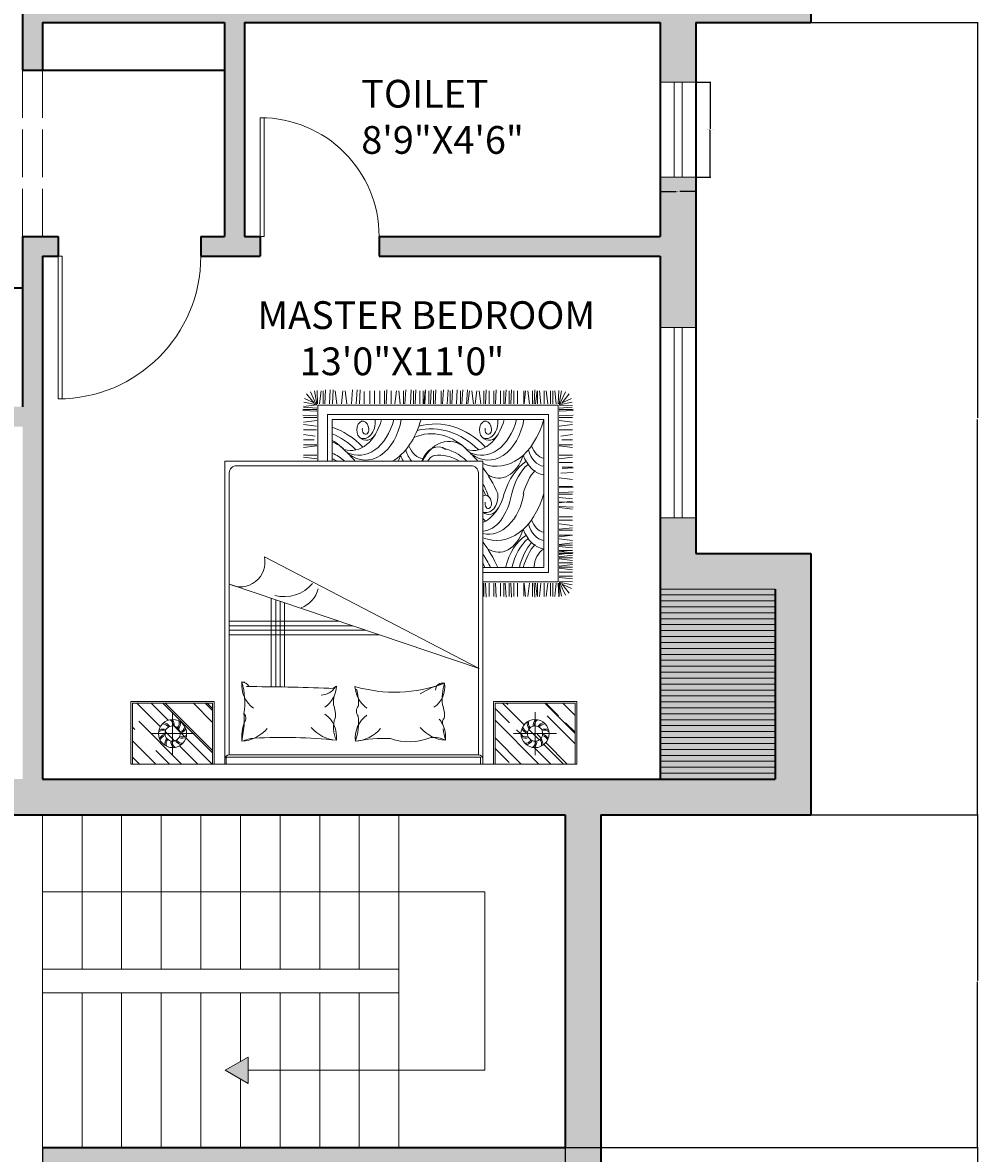
# Model space of a CAD drawing. Units: inches. Extents: x 2540 to 3167, y 3083 to 4007.
# Tile 14 of 15: x 2926 to 3167, y 3542 to 3828. Entities that reach past the tile are written whole.
import ezdxf

# ---------------------------------------------------------------- set-up
doc = ezdxf.new("R2010")
doc.units = ezdxf.units.IN
doc.linetypes.add('ACAD_ISO02W100', pattern=[15, 12, -3])
for name, color, linetype, lineweight in [('A-ANNO-DIMS', 2, 'Continuous', 18), ('A-ANNO-SYMB', 7, 'Continuous', 18), ('A-AREA-IDEN', 7, 'Continuous', 18), ('A-DOOR', 4, 'Continuous', 18), ('A-FLOR-PATT', 8, 'Continuous', 13), ('A-FLOR-STRS', 7, 'Continuous', 18), ('A-FURN', 8, 'Continuous', 13), ('A-GLAZ', 4, 'Continuous', 18)]:
    doc.layers.add(name, color=color, linetype=linetype, lineweight=lineweight)
for name, color, linetype, lineweight, true_color in [('A-WALL', 143, 'Continuous', 35, 0x7aafdf), ('A-WALL-OVHD', 143, 'ACAD_ISO02W100', 18, 0x7aafdf), ('A-WALL-PATT', 143, 'Continuous', 13, 0x7aafdf)]:
    doc.layers.add(name, color=color, linetype=linetype, lineweight=lineweight, true_color=true_color)
doc.styles.get("Standard").update_dxf_attribs({"font": 'arial.ttf'})
doc.dimstyles.get("Standard").update_dxf_attribs({"dimtxt": 0.18, "dimasz": 0.18, "dimexe": 0.18, "dimexo": 0.0625, "dimgap": 0.09, "dimtad": 0, "dimtih": 1, "dimtoh": 1, "dimdec": 4, "dimzin": 0, "dimdsep": 46, "dimtxsty": 'Standard', "dimcen": 0.09, "dimadec": 0, "dimazin": 0, "dimtfac": 1, "dimtdec": 4, "dimtofl": 0, "dimtmove": 0, "dimatfit": 3, "dimfxl": 1, "dimtolj": 1, "dimtzin": 0, "dimarcsym": 0})

# ---------------------------------------------------------------- blocks, each defined once
blk = doc.blocks.new('*U3')
blk.add_line((0, 0), (0, 29))
blk = doc.blocks.new('*U4')
at = {"layer": 'A-FLOR-PATT', "color": 0, "linetype": 'ByBlock', "lineweight": -2, "transparency": 16777216, "rotation": 270}
for p in [(3086.51, 3684.71), (3086.51, 3683.21), (3086.51, 3681.71), (3086.51, 3680.21), (3086.51, 3678.71), (3086.51, 3677.21), (3086.51, 3675.71), (3086.51, 3674.21), (3086.51, 3672.71), (3086.51, 3671.21), (3086.51, 3669.71), (3086.51, 3668.21), (3086.51, 3666.71), (3086.51, 3665.21), (3086.51, 3663.71), (3086.51, 3662.21), (3086.51, 3660.71), (3086.51, 3659.21), (3086.51, 3657.71), (3086.51, 3656.21), (3086.51, 3654.71), (3086.51, 3653.21), (3086.51, 3651.71), (3086.51, 3650.21), (3086.51, 3648.71), (3086.51, 3647.21), (3086.51, 3645.71), (3086.51, 3644.21), (3086.51, 3642.71), (3086.51, 3641.21), (3086.51, 3639.71), (3086.51, 3638.21), (3086.51, 3636.71)]:
    blk.add_blockref('*U3', p, dxfattribs=at)
blk = doc.blocks.new('A$C64B41DC1')
for p, q in [((0, 2.5079), (2.9903, 2.5079)), ((0, 2.0879), (0, 2.5079)), ((0.012, 2.4618), (0.0581, 2.5079)), ((0.012, 2.3515), (0.1684, 2.5079)), ((0.012, 2.0999), (0.012, 2.5079)), ((0.0543, 2.2213), (0.3409, 2.5079)), ((0.1689, 2.4179), (0.2589, 2.5079)), ((0.3265, 2.386), (0.4484, 2.5079)), ((0.3699, 2.3332), (0.5445, 2.5079)), ((0.548, 2.5079), (0.548, 2.0999)), ((0.56, 2.5079), (0.56, 2.0879)), ((0.6301, 2.5079), (0.6301, 0.4779)), ((0.6401, 2.461), (0.6401, 2.5079)), ((0.6401, 2.5079), (2.344, 2.5079)), ((2.344, 2.5079), (2.3601, 2.5079)), ((2.344, 2.5079), (2.344, 2.461)), ((2.3601, 2.5079), (2.3601, 2.4761)), ((2.3601, 0.4779), (2.3601, 2.5079)), ((2.4303, 2.5079), (2.4303, 2.0879)), ((2.4423, 2.5079), (2.4423, 2.0999)), ((2.4423, 2.3333), (2.6169, 2.5079)), ((2.4423, 2.2145), (2.7357, 2.5079)), ((2.705, 2.398), (2.8149, 2.5079)), ((2.7691, 2.3772), (2.8998, 2.5079)), ((2.7819, 2.3646), (2.9252, 2.5079)), ((2.9783, 2.0999), (2.9783, 2.5079)), ((2.9903, 2.0879), (2.9903, 2.5079)), ((0.2157, 2.0999), (0.548, 2.4322)), ((0.2804, 2.1597), (0.2804, 2.4481)), ((2.344, 2.461), (0.6401, 2.461)), ((0.6601, 2.4461), (1.4951, 2.4461)), ((0.6601, 2.4461), (0.6601, 0.5579)), ((1.4951, 2.4461), (0.6697, 2.4461)), ((2.3301, 2.4461), (1.4951, 2.4461)), ((2.3301, 0.5579), (2.3301, 2.4461)), ((2.4423, 2.404), (2.5354, 2.4971)), ((2.7099, 2.1597), (2.7099, 2.4481)), ((0.2299, 2.0999), (0.548, 2.418)), ((0.2311, 2.2906), (0.2937, 2.3532)), ((2.7914, 2.1846), (2.9783, 2.3715)), ((0.012, 2.261), (0.0275, 2.2765)), ((0.1362, 2.3039), (0.4246, 2.3039)), ((0.2905, 2.2539), (0.3304, 2.2938)), ((0.3405, 2.3039), (0.3605, 2.3238)), ((2.8541, 2.3039), (2.5657, 2.3039)), ((2.5849, 2.2779), (2.6158, 2.3088)), ((2.6158, 2.3088), (2.6313, 2.3243)), ((2.6674, 2.2756), (2.7382, 2.3464)), ((2.7249, 2.3076), (2.7512, 2.3339)), ((2.7746, 2.0999), (2.9783, 2.3036)), ((2.9144, 2.2312), (2.9783, 2.2951)), ((0.0404, 2.0999), (0.1982, 2.2578)), ((0.1365, 2.0999), (0.251, 2.2144)), ((0.4194, 2.0999), (0.548, 2.2285)), ((2.4423, 2.1353), (2.5382, 2.2312)), ((2.4918, 2.0999), (2.6366, 2.2447)), ((0.4986, 2.0999), (0.548, 2.1493)), ((0.5127, 2.0999), (0.548, 2.1352)), ((2.7831, 2.0999), (2.8678, 2.1846)), ((2.8962, 2.0999), (2.9783, 2.182)), ((0.56, 2.0879), (0, 2.0879)), ((0.548, 2.0999), (0.012, 2.0999)), ((2.4303, 2.0879), (2.9903, 2.0879)), ((2.4423, 2.0999), (2.9783, 2.0999)), ((2.5172, 2.0999), (2.5269, 2.1096)), ((0.9415, 1.9902), (0.9415, 1.3975)), ((0.9715, 1.9906), (0.9715, 1.4076)), ((1.0015, 1.991), (1.0015, 1.4177)), ((1.0315, 1.9916), (1.0315, 1.4279)), ((2.3349, 1.8678), (0.6613, 1.3029)), ((0.8956, 1.1191), (2.3349, 1.8678)), ((1.6636, 1.6412), (0.6601, 1.6412)), ((1.5748, 1.6112), (0.6601, 1.6112)), ((2.3665, 1.295), (2.3665, 1.3839)), ((2.377, 1.295), (2.3822, 1.3891)), ((2.4032, 1.295), (2.4032, 1.3839)), ((2.4346, 1.295), (2.4346, 1.3839)), ((2.4451, 1.295), (2.4503, 1.3891)), ((2.4774, 1.2957), (2.4774, 1.3837)), ((2.5, 1.295), (2.5, 1.3839)), ((2.5105, 1.295), (2.5157, 1.3891)), ((2.5367, 1.295), (2.5367, 1.3839)), ((2.5471, 1.295), (2.5524, 1.3891)), ((2.5681, 1.295), (2.5681, 1.3839)), ((2.5918, 1.295), (2.5918, 1.3839)), ((2.6346, 1.2957), (2.6346, 1.3837)), ((2.6362, 1.2957), (2.6467, 1.3839)), ((2.6729, 1.295), (2.6624, 1.3839)), ((2.6938, 1.295), (2.6938, 1.3839)), ((2.7043, 1.295), (2.7095, 1.3891)), ((2.7127, 1.2957), (2.7232, 1.3839)), ((2.7253, 1.295), (2.7253, 1.3839)), ((2.7494, 1.295), (2.7389, 1.3839)), ((2.7718, 1.295), (2.7718, 1.3839)), ((2.7959, 1.295), (2.7854, 1.3839)), ((2.8146, 1.2957), (2.8146, 1.3837)), ((2.8146, 1.2957), (2.8146, 1.3837)), ((2.8282, 1.295), (2.8282, 1.3839)), ((2.8282, 1.295), (2.8282, 1.3839)), ((2.8523, 1.295), (2.8418, 1.3839)), ((2.8523, 1.295), (2.8418, 1.3839)), ((2.8653, 1.2966), (2.8688, 1.3861)), ((2.8711, 1.2957), (2.8711, 1.3837)), ((2.8711, 1.2957), (2.8875, 1.3822)), ((2.8765, 1.2958), (2.9132, 1.3758)), ((2.8713, 1.2927), (2.954, 1.3315)), ((2.8717, 1.2884), (2.9588, 1.3058)), ((2.8893, 1.3011), (2.9394, 1.3636)), ((2.3601, 1.2873), (2.8639, 1.2873)), ((2.3601, 1.2233), (2.7999, 1.2233)), ((2.7999, 1.2233), (2.7999, 0.1658)), ((2.8639, 1.2873), (2.8639, 0.1018)), ((2.8716, 1.2565), (2.9605, 1.2669)), ((2.8716, 1.2212), (2.9605, 1.2212)), ((2.8723, 1.2489), (2.9603, 1.2489)), ((2.8744, 1.2817), (2.9603, 1.2869)), ((2.3601, 1.1913), (2.7679, 1.1912)), ((2.7679, 1.1912), (2.7679, 0.1978)), ((2.8716, 1.1947), (2.9605, 1.2052)), ((2.8716, 1.181), (2.9605, 1.1705)), ((2.8716, 1.1595), (2.9605, 1.1595)), ((2.8716, 1.133), (2.9605, 1.1435)), ((2.8723, 1.1872), (2.9603, 1.1872)), ((2.8716, 1.1193), (2.9605, 1.1088)), ((2.8716, 1.1035), (2.9605, 1.093)), ((2.8716, 1.0965), (2.9605, 1.0965)), ((2.8716, 1.086), (2.9657, 1.0913)), ((2.8716, 1.0756), (2.9605, 1.0756)), ((2.8723, 1.1255), (2.9603, 1.1255)), ((2.8723, 1.0858), (2.9605, 1.0753)), ((2.8716, 1.0491), (2.9605, 1.0596)), ((2.8716, 1.0354), (2.9605, 1.0249)), ((2.8723, 1.0416), (2.9603, 1.0416)), ((2.8723, 0.9987), (2.9605, 1.0092)), ((2.8716, 0.9346), (2.9605, 0.9241)), ((2.8723, 0.985), (2.9605, 0.9745)), ((2.8723, 0.9735), (2.9603, 0.9735)), ((2.8723, 0.9408), (2.9603, 0.9408)), ((2.8723, 0.8979), (2.9605, 0.9084)), ((2.8723, 0.8726), (2.9603, 0.8726)), ((2.8723, 0.8505), (2.9603, 0.8505)), ((2.8716, 0.7885), (2.9605, 0.799)), ((2.8716, 0.7818), (2.9657, 0.787)), ((2.8716, 0.7503), (2.9657, 0.7556)), ((2.8716, 0.7204), (2.9605, 0.7309)), ((2.8716, 0.6995), (2.9605, 0.6995)), ((2.8716, 0.689), (2.9657, 0.6838)), ((2.8723, 0.7571), (2.9605, 0.7466)), ((2.8716, 0.6576), (2.9657, 0.6523)), ((2.8716, 0.6471), (2.9605, 0.6471)), ((2.8716, 0.5903), (2.9605, 0.6007)), ((2.882, 0.5582), (2.9657, 0.5536)), ((0.6301, 0.4779), (2.3601, 0.4779)), ((0.7101, 0.5079), (2.2801, 0.5079)), ((1.2465, 0.4625), (1.1576, 0.452)), ((1.2542, 0.1018), (1.2542, 0.4779)), ((1.3182, 0.1658), (1.3182, 0.4779)), ((1.3502, 0.1978), (1.3502, 0.4779)), ((2.8716, 0.4877), (2.9603, 0.4877)), ((2.8716, 0.4625), (2.9605, 0.452)), ((2.8909, 0.5263), (2.9657, 0.5222)), ((2.8928, 0.5169), (2.9605, 0.5169)), ((1.2465, 0.3746), (1.1576, 0.3851)), ((1.2465, 0.4365), (1.1577, 0.4365)), ((2.8716, 0.4365), (2.9603, 0.4365)), ((2.8716, 0.3746), (2.9605, 0.3851)), ((1.2355, 0.3092), (1.1576, 0.3)), ((1.2465, 0.3684), (1.1577, 0.3684)), ((1.2285, 0.3357), (1.1577, 0.3357)), ((2.8716, 0.3684), (2.9603, 0.3684)), ((2.8826, 0.3092), (2.9605, 0.3)), ((2.8896, 0.3357), (2.9603, 0.3357)), ((1.2457, 0.2423), (1.1576, 0.2319)), ((1.2457, 0.2676), (1.1577, 0.2676)), ((2.8723, 0.2676), (2.9603, 0.2676)), ((2.8723, 0.2423), (2.9605, 0.2319)), ((1.2465, 0.1742), (1.1524, 0.169)), ((1.2465, 0.2057), (1.1576, 0.2161)), ((1.2465, 0.1847), (1.1576, 0.1847)), ((2.7999, 0.1658), (1.3182, 0.1658)), ((2.7679, 0.1978), (1.3502, 0.1978)), ((2.8716, 0.2057), (2.9605, 0.2161)), ((2.8716, 0.1847), (2.9605, 0.1847)), ((2.8716, 0.1742), (2.9657, 0.169)), ((1.2465, 0.1428), (1.1524, 0.1376)), ((1.2465, 0.1334), (1.1524, 0.1281)), ((1.2465, 0.1323), (1.1576, 0.1323)), ((1.2465, 0.1323), (1.1576, 0.1323)), ((1.2465, 0.1), (1.1576, 0.1105)), ((1.2465, 0.1229), (1.1588, 0.1168)), ((1.2464, 0.1007), (1.1592, 0.0833)), ((1.2468, 0.0964), (1.1641, 0.0576)), ((1.2288, 0.088), (1.1787, 0.0255)), ((1.2415, 0.0933), (1.2049, 0.0133)), ((1.247, 0.0934), (1.2306, 0.0069)), ((1.2527, 0.0925), (1.2493, 0.003)), ((2.8639, 0.1018), (1.2542, 0.1018)), ((1.2658, 0.0941), (1.2762, 0.0052)), ((1.2899, 0.0941), (1.2899, 0.0052)), ((1.2999, 0.0941), (1.3051, 0)), ((1.3313, 0.0941), (1.3365, 0)), ((1.3523, 0.0941), (1.3575, 0)), ((1.3804, 0.0941), (1.3699, 0.0052)), ((1.4119, 0.0934), (1.4223, 0.0052)), ((1.4485, 0.0941), (1.438, 0.0052)), ((1.48, 0.0941), (1.4852, 0)), ((1.5114, 0.0941), (1.5166, 0)), ((1.5323, 0.0941), (1.5376, 0)), ((1.5638, 0.0941), (1.5638, 0.0105)), ((1.6021, 0.0941), (1.6021, 0.0052)), ((1.6336, 0.0941), (1.6336, 0.0052)), ((1.6702, 0.0941), (1.6702, 0.0052)), ((1.7017, 0.0941), (1.7017, 0.0052)), ((1.7122, 0.0941), (1.7174, 0)), ((1.7445, 0.0934), (1.7445, 0.0054)), ((1.7698, 0.0934), (1.7803, 0.0052)), ((1.8065, 0.0941), (1.796, 0.0052)), ((1.8274, 0.0941), (1.8274, 0.0052)), ((1.8379, 0.0941), (1.8431, 0)), ((1.8746, 0.0941), (1.8798, 0)), ((1.8955, 0.0941), (1.8955, 0.0052)), ((1.906, 0.0941), (1.9113, 0)), ((1.9384, 0.0934), (1.9384, 0.0054)), ((1.9609, 0.0941), (1.9609, 0.0052)), ((1.9636, 0.0934), (1.9741, 0.0052)), ((1.9714, 0.0941), (1.9766, 0)), ((1.9976, 0.0941), (1.9976, 0.0052)), ((2.0081, 0.0941), (2.0133, 0)), ((2.029, 0.0941), (2.029, 0.0052)), ((2.0395, 0.0941), (2.0447, 0)), ((2.0797, 0.0941), (2.0797, 0.0052)), ((2.0902, 0.0941), (2.0954, 0)), ((2.1216, 0.0941), (2.1269, 0)), ((2.1412, 0.0941), (2.1412, 0.0052)), ((2.1517, 0.0941), (2.1569, 0)), ((2.1831, 0.0941), (2.1884, 0)), ((2.2093, 0.0941), (2.2093, 0.0052)), ((2.2198, 0.0941), (2.225, 0)), ((2.2512, 0.0941), (2.2565, 0)), ((2.2603, 0.0934), (2.2707, 0.0052)), ((2.2969, 0.0941), (2.2864, 0.0052)), ((2.3089, 0.0934), (2.3193, 0.0052)), ((2.3455, 0.0941), (2.3351, 0.0052)), ((2.3665, 0.0941), (2.3665, 0.0052)), ((2.377, 0.0941), (2.3822, 0)), ((2.4032, 0.0941), (2.4032, 0.0052)), ((2.4346, 0.0941), (2.4346, 0.0052)), ((2.4451, 0.0941), (2.4503, 0)), ((2.4774, 0.0934), (2.4774, 0.0054)), ((2.5, 0.0941), (2.5, 0.0052)), ((2.5105, 0.0941), (2.5157, 0)), ((2.5367, 0.0941), (2.5367, 0.0052)), ((2.5471, 0.0941), (2.5524, 0)), ((2.5681, 0.0941), (2.5681, 0.0052)), ((2.5918, 0.0941), (2.5918, 0.0052)), ((2.6346, 0.0934), (2.6346, 0.0054)), ((2.6362, 0.0934), (2.6467, 0.0052)), ((2.6729, 0.0941), (2.6624, 0.0052)), ((2.6938, 0.0941), (2.6938, 0.0052)), ((2.7043, 0.0941), (2.7095, 0)), ((2.7127, 0.0934), (2.7232, 0.0052)), ((2.7253, 0.0941), (2.7253, 0.0052)), ((2.7494, 0.0941), (2.7389, 0.0052)), ((2.7718, 0.0941), (2.7718, 0.0052)), ((2.7959, 0.0941), (2.7854, 0.0052)), ((2.8146, 0.0934), (2.8146, 0.0054)), ((2.8282, 0.0941), (2.8282, 0.0052)), ((2.8523, 0.0941), (2.8418, 0.0052)), ((2.8653, 0.0925), (2.8688, 0.003)), ((2.8711, 0.0934), (2.8875, 0.0069)), ((2.8713, 0.0964), (2.954, 0.0576)), ((2.8716, 0.1428), (2.9657, 0.1376)), ((2.8716, 0.1334), (2.9657, 0.1281)), ((2.8716, 0.1323), (2.9605, 0.1323)), ((2.8716, 0.1229), (2.9593, 0.1168)), ((2.8717, 0.1007), (2.9588, 0.0833)), ((2.8744, 0.1074), (2.9603, 0.1022)), ((2.8765, 0.0933), (2.9132, 0.0133)), ((2.8893, 0.088), (2.9394, 0.0255))]:
    blk.add_line(p, q)
at = {"ltscale": 10}
for p, q in [((1.4859, 1.5812), (0.6601, 1.5812)), ((1.397, 1.5512), (0.6601, 1.5512))]:
    blk.add_line(p, q, dxfattribs=at)
for centre, radius in [((0.2804, 2.3039), 0.0942), ((0.2804, 2.3039), 0.051), ((2.7099, 2.3039), 0.0942), ((2.7099, 2.3039), 0.051)]:
    blk.add_circle(centre, radius)
for centre, radius, start, end in [((0.6601, 2.4761), 0.03, 180, 270), ((2.3301, 2.4761), 0.03, 270, 0), ((0.2887, 2.3745), 0.0605, 172.17003, 218.48975), ((0.2828, 2.3731), 0.0462, 160.30017, 220.53802), ((0.3286, 2.3561), 0.0605, 136.17003, 182.48975), ((0.3231, 2.3585), 0.0462, 124.30017, 184.53802), ((0.3501, 2.3178), 0.0605, 100.17003, 146.48975), ((0.347, 2.323), 0.0462, 88.30017, 148.53802), ((1.0526, 2.3302), 0.3085, 175.30484, 198.69419), ((-0.8702, 2.0941), 1.6364, 4.80985, 9.18918), ((0.8579, 2.6278), 0.2948, 247.51785, 264.26696), ((0.728, 2.111), 0.245, 40.4189, 85.9871), ((1.6986, 2.3355), 0.1943, 174.11002, 233.4289), ((1.1481, 2.2311), 0.3783, 353.49469, 19.18669), ((1.6871, 3.192), 0.8561, 257.74383, 273.62843), ((1.4882, 2.111), 0.245, 40.4189, 85.9871), ((1.8674, 1.9709), 0.3878, 68.20259, 108.9817), ((2.6433, 2.323), 0.0462, 31.46198, 91.69983), ((2.6402, 2.3178), 0.0605, 33.51025, 79.82997), ((2.6672, 2.3585), 0.0462, 355.46198, 55.69983), ((2.6617, 2.3561), 0.0605, 357.51025, 43.82997), ((2.7075, 2.3731), 0.0462, 319.46198, 19.69983), ((2.7016, 2.3745), 0.0605, 321.51025, 7.82997), ((0.2153, 2.3276), 0.0462, 232.30017, 292.53802), ((0.2158, 2.3336), 0.0605, 244.17003, 290.48975), ((0.2457, 2.3659), 0.0605, 208.17003, 254.48975), ((0.2417, 2.3614), 0.0462, 196.30017, 256.53802), ((0.3449, 2.2742), 0.0605, 64.17003, 110.48975), ((0.3455, 2.2802), 0.0462, 52.30017, 112.53802), ((0.3191, 2.2464), 0.0462, 16.30017, 76.53802), ((0.3151, 2.2419), 0.0605, 28.17003, 74.48975), ((1.0164, 5.7096), 3.3803, 266.81337, 276.16021), ((1.3963, 2.1044), 0.245, 94.0129, 139.5811), ((1.1858, 2.3288), 0.1943, 306.5711, 5.88998), ((1.5348, 2.2652), 0.1767, 151.77364, 201.69827), ((2.1269, 2.1044), 0.245, 94.0129, 139.5811), ((2.0342, 2.4856), 0.1563, 261.59582, 298.90918), ((1.9165, 2.3288), 0.1943, 333.73715, 5.88998), ((2.6058, 2.2028), 0.517, 163.60457, 172.3273), ((2.6448, 2.2802), 0.0462, 67.46198, 127.69983), ((2.6454, 2.2742), 0.0605, 69.51025, 115.82997), ((2.6752, 2.2419), 0.0605, 105.51025, 151.82997), ((2.6712, 2.2464), 0.0462, 103.46198, 163.69983), ((2.7744, 2.3336), 0.0605, 249.51025, 295.82997), ((2.775, 2.3276), 0.0462, 247.46198, 307.69983), ((2.7486, 2.3614), 0.0462, 283.46198, 343.69983), ((2.7446, 2.3659), 0.0605, 285.51025, 331.82997), ((0.2138, 2.2848), 0.0462, 268.30017, 328.53802), ((0.2107, 2.29), 0.0605, 280.17003, 326.48975), ((0.2377, 2.2493), 0.0462, 304.30017, 4.53802), ((0.2322, 2.2517), 0.0605, 316.17003, 2.48975), ((0.2779, 2.2347), 0.0462, 340.30017, 40.53802), ((0.272, 2.2333), 0.0605, 352.17003, 38.48975), ((0.7274, 2.2013), 0.0446, 314.4736, 42.17134), ((-1.6008, 2.277), 2.3618, 357.39054, 358.88764), ((1.204, 2.1778), 0.1681, 337.01697, 7.53676), ((1.9165, 2.3288), 0.1943, 320.94042, 333.73715), ((2.1347, 2.2313), 0.0459, 165.35061, 223.26844), ((1.9346, 2.1778), 0.1681, 337.01697, 7.53676), ((2.7182, 2.2333), 0.0605, 141.51025, 187.82997), ((2.7123, 2.2347), 0.0462, 139.46198, 199.69983), ((2.7581, 2.2517), 0.0605, 177.51025, 223.82997), ((2.7526, 2.2493), 0.0462, 175.46198, 235.69983), ((2.7796, 2.29), 0.0605, 213.51025, 259.82997), ((2.7765, 2.2848), 0.0462, 211.46198, 271.69983), ((0.9385, 1.978), 0.1943, 126.5711, 185.88998), ((0.2688, 2.0945), 0.4956, 344.0243, 8.70709), ((1.1858, 1.9714), 0.1943, 4.31813, 53.4289), ((1.7059, 1.9714), 0.204, 127.11975, 175.09005), ((1.5671, 2.1546), 0.0547, 142.08329, 220.902), ((1.9394, 1.991), 0.1651, 351.26213, 55.75721), ((1.2687, 1.9248), 0.1223, 33.62799, 86.47438), ((1.5415, 2.0969), 0.1834, 175.22328, 196.23004), ((1.1965, 2.0983), 0.3299, 343.79543, 3.55541), ((2.4617, 2.0719), 0.3745, 173.82958, 196.4356), ((0.7417, 2.0149), 0.057, 273.47085, 328.54118), ((0.7246, 18.8439), 16.8552, 270.17399, 272.05214), ((1.3401, 1.9404), 0.0603, 49.09906, 101.37023), ((1.7676, 1.0629), 0.9631, 69.65065, 105.96307), ((2.2748, 2.5795), 0.6373, 238.34989, 254.31375), ((2.0911, 2.0123), 0.0478, 179.77267, 283.80184), ((0.728, 2.2025), 0.245, 274.0129, 278.34166), ((1.0747, 1.2871), 0.1871, 14.1863, 69.12121), ((1.0274, 1.1334), 0.2527, 40.62904, 104.37123), ((0.7347, 1.1553), 0.1649, 347.31088, 116.44537), ((0.7101, 0.5579), 0.05, 180, 270), ((2.2801, 0.5579), 0.05, 270, 0)]:
    blk.add_arc(centre, radius, start, end)
for centre, major_axis, ratio, start_param, end_param in [((1.9938, 1.6262), (0, -0.7531), 0.68, 0.797284, 0.954936), ((2.0643, 1.466), (0, -0.5322), 0.68, 7.239912, 7.311536), ((1.9052, 1.7397), (0, -0.9842), 0.68, 0.74745, 0.979724), ((2.7455, 1.3081), (0, 0.3614), 0.68, 1.900046, 2.742661), ((2.7868, 1.3081), (0, 0.3614), 0.68, 1.900046, 2.614747), ((2.8372, 1.3081), (0, 0.3614), 0.68, 1.900046, 2.479658), ((2.8607, 1.3211), (0, 0.3614), 0.68, 1.938265, 2.479658), ((2.8057, 1.2079), (0, -0.1524), 0.68, 4.821745, 5.895886), ((2.4665, 0.8216), (0, -0.2664), 0.68, 2.006169, 3.565187), ((2.7862, 0.8069), (0, -0.2615), 0.68, 3.244645, 4.205018), ((2.4513, 0.5069), (0, 0.502), 0.68, 5.095327, 6.553458), ((2.396, 0.6032), (0, 0.3641), 0.68, -1.3172, 0.145284), ((2.7784, 0.8289), (0, -0.1802), 0.68, 3.227058, 4.318474), ((2.3507, 0.5642), (0.0073, 0.3819), 0.56205, -1.21172, -0.009991), ((2.7821, 0.7971), (0, -0.1589), 0.68, 3.272942, 4.229533), ((2.2964, 0.5771), (0, -0.3263), 0.68, 1.938944, 2.850232), ((2.0403, 1.6015), (0, -0.8763), 0.68, 6.849801, 6.887077), ((2.4005, 0.7132), (0, -0.1214), 0.68, 2.284368, 3.652258), ((2.3834, 0.7081), (0, 0.1147), 0.68, 4.593909, 6.585576), ((2.3774, 0.7653), (0, -0.0593), 0.68, 5.841311, 7.755362), ((2.3961, 0.7628), (0, -0.0317), 0.68, 1.462497, 5.046281), ((1.9938, 1.1295), (-0.0678, 0.7439), 0.610498, 3.917146, 4.063997), ((2.0643, 0.9693), (0, -0.5322), 0.68, 7.239912, 7.336618), ((1.9052, 1.243), (0, -0.9842), 0.68, 0.74745, 0.979724), ((2.7455, 0.8114), (-0.0599, 0.3735), 0.695517, 1.775813, 2.548612), ((2.7868, 0.8114), (0, 0.3614), 0.68, 1.900046, 2.614747), ((2.8607, 0.8243), (0, 0.3614), 0.68, 1.938265, 2.479658), ((2.4665, 0.3249), (0, -0.2664), 0.68, 2.006169, 3.565187), ((2.4513, 0.0102), (0, 0.502), 0.68, 5.095327, 6.553458), ((2.7862, 0.3102), (0, -0.2615), 0.68, 3.244645, 4.205018), ((1.242, 0.9693), (0, -0.5322), 0.68, 6.586764, 6.677612), ((1.1714, 1.1295), (-0.1157, 0.7241), 0.59432, 3.291697, 3.50733), ((1.0828, 1.243), (0, -0.9842), 0.68, 0.565948, 0.680366), ((1.5283, 0.0674), (0, -0.3703), 0.68, 1.930561, 3.464283), ((1.5736, 0.1065), (0, 0.3641), 0.68, -1.3172, 0.476403), ((1.6289, 0.0102), (0, 0.502), 0.68, 6.655152, 6.661293), ((1.6289, 0.0102), (0, 0.502), 0.68, 5.095327, 5.911219), ((1.6442, 0.3249), (0, -0.2664), 0.68, 2.006169, 2.182797), ((1.9638, 0.3102), (0, -0.2615), 0.68, 4.015924, 4.205018), ((1.956, 0.3322), (0, -0.1802), 0.68, 3.770744, 4.318474), ((1.9597, 0.3004), (0, -0.1589), 0.68, 3.14258, 4.229533), ((2.0606, 0.5616), (0, -0.1803), 0.68, 5.194792, 5.929328), ((2.0606, 0.5616), (0, -0.1803), 0.68, 5.194792, 6.723255), ((2.1315, 0.6603), (0, -0.3155), 0.68, 5.328638, 6.949396), ((2.0549, 0.5656), (0, -0.1303), 0.68, 5.450951, 6.054641), ((2.0643, 0.9693), (0, -0.5322), 0.68, 6.20013, 6.677612), ((1.9938, 1.1295), (-0.0678, 0.7439), 0.610498, 3.199135, 3.592282), ((1.9052, 1.243), (0, -0.9842), 0.68, 0.565948, 0.680366), ((2.3507, 0.0674), (0, -0.3703), 0.68, 1.930561, 3.464283), ((2.396, 0.1065), (0, 0.3641), 0.68, -1.3172, 0.476403), ((2.4513, 0.0102), (0, 0.502), 0.68, 6.655152, 6.661293), ((2.7784, 0.3322), (0, -0.1802), 0.68, 3.227058, 4.318474), ((2.7821, 0.3004), (0, -0.1589), 0.68, 3.272942, 4.229533), ((1.1933, 0.9181), (0, -0.624), 0.68, 0.378672, 0.625379), ((1.3091, 0.6603), (0, -0.3155), 0.68, 6.475719, 6.949396), ((1.1911, 1.1066), (0, 0.8458), 0.68, 3.421828, 3.728616), ((1.2179, 1.1047), (0, -0.8763), 0.68, 6.507006, 6.887077), ((1.474, 0.0804), (0, -0.3263), 0.68, 1.938944, 3.339184), ((2.0157, 0.9181), (0, -0.624), 0.68, -0.280078, 0.625379), ((2.0135, 1.1066), (0, 0.8458), 0.68, 2.978727, 3.728616), ((2.0403, 1.1047), (0, -0.8763), 0.68, 6.099302, 6.887077), ((2.2964, 0.0804), (0, -0.3263), 0.68, 1.938944, 3.339184), ((1.555, 0.2685), (0, -0.0593), 0.68, 3.732151, 7.755362), ((1.5781, 0.2165), (0, -0.1214), 0.68, 2.284368, 3.726131), ((1.561, 0.2114), (0, 0.1147), 0.68, 4.593909, 6.647252), ((2.3774, 0.2685), (0, -0.0593), 0.68, 3.732151, 7.755362), ((2.4005, 0.2165), (0, -0.1214), 0.68, 2.284368, 3.726131), ((2.3834, 0.2114), (0, 0.1147), 0.68, 4.593909, 6.647252), ((1.5737, 0.2661), (0, -0.0317), 0.68, 1.462497, 5.046281), ((2.3961, 0.2661), (0, -0.0317), 0.68, 1.462497, 5.046281)]:
    blk.add_ellipse(centre, major_axis=major_axis, ratio=ratio, start_param=start_param, end_param=end_param)
blk = doc.blocks.new('DOOR-SWING-30IN')
for p, q in [((0, 0), (0, 30)), ((1, 0), (1, 29.98)), ((0, 0), (1, 0))]:
    blk.add_line(p, q)
blk.add_arc((0, 0), 30, 0, 90)
blk = doc.blocks.new('WIN-24IN')
for p, q in [((0, 24), (9, 24)), ((3.5, 0), (3.5, 24)), ((5.5, 0), (5.5, 24)), ((0, 0), (9, 0))]:
    blk.add_line(p, q)
blk = doc.blocks.new('WIN-48IN')
for p, q in [((0, 48), (9, 48)), ((3.5, 0), (3.5, 48)), ((5.5, 0), (5.5, 48)), ((0, 0), (9, 0))]:
    blk.add_line(p, q)
blk = doc.blocks.new('*D29')
at = {"layer": 'A-ANNO-DIMS', "color": 0, "lineweight": -2, "transparency": 16777216}
for p, q in [((3095.57, 3812.71), (3099.29, 3812.71)), ((3099.11, 3812.53), (3099.11, 3800.9)), ((3099.11, 3788.89), (3099.11, 3800.53)), ((3095.57, 3788.71), (3099.29, 3788.71))]:
    blk.add_line(p, q, dxfattribs=at)
at = {"layer": 'A-ANNO-DIMS', "color": 0, "transparency": 16777216}
for points in [[(3099.08, 3812.53), (3099.14, 3812.53), (3099.11, 3812.71)], [(3099.08, 3788.89), (3099.14, 3788.89), (3099.11, 3788.71)]]:
    blk.add_solid(points, dxfattribs=at)
at = {"layer": 'Defpoints', "color": 0, "transparency": 16777216}
for p in [(3095.51, 3812.71), (3099.11, 3812.71), (3095.51, 3788.71)]:
    blk.add_point(p, dxfattribs=at)
at = {"layer": 'A-ANNO-DIMS', "color": 0, "transparency": 16777216, "insert": (3099.11, 3800.71), "char_height": 0.18, "attachment_point": 5}
blk.add_mtext('\\A1;WINDOW 24 TYP.', dxfattribs=at)
blk = doc.blocks.new('*D30')
at = {"layer": 'A-ANNO-DIMS', "color": 0, "lineweight": -2, "transparency": 16777216}
for p, q in [((3086.51, 3788.65), (3086.51, 3784.93)), ((3095.51, 3788.65), (3095.51, 3784.93)), ((3086.69, 3785.11), (3090.55, 3785.11)), ((3095.33, 3785.11), (3091.47, 3785.11))]:
    blk.add_line(p, q, dxfattribs=at)
at = {"layer": 'A-ANNO-DIMS', "color": 0, "transparency": 16777216}
for points in [[(3086.69, 3785.14), (3086.69, 3785.08), (3086.51, 3785.11)], [(3095.33, 3785.14), (3095.33, 3785.08), (3095.51, 3785.11)]]:
    blk.add_solid(points, dxfattribs=at)
at = {"layer": 'Defpoints', "color": 0, "transparency": 16777216}
for p in [(3086.51, 3788.71), (3095.51, 3788.71), (3095.51, 3785.11)]:
    blk.add_point(p, dxfattribs=at)
at = {"layer": 'A-ANNO-DIMS', "color": 0, "transparency": 16777216, "insert": (3091.01, 3785.11), "char_height": 0.18, "attachment_point": 5}
blk.add_mtext('\\A1;9 TYP.', dxfattribs=at)
blk = doc.blocks.new('*D49')
at = {"layer": 'A-ANNO-DIMS', "color": 0, "lineweight": -2, "transparency": 16777216}
for p, q in [((3124.57, 3827.71), (3166.79, 3827.71)), ((3166.61, 3827.53), (3166.61, 3727.9)), ((3166.61, 3627.89), (3166.61, 3727.53)), ((3124.57, 3627.71), (3166.79, 3627.71))]:
    blk.add_line(p, q, dxfattribs=at)
at = {"layer": 'A-ANNO-DIMS', "color": 0, "transparency": 16777216}
for points in [[(3166.58, 3827.53), (3166.64, 3827.53), (3166.61, 3827.71)], [(3166.58, 3627.89), (3166.64, 3627.89), (3166.61, 3627.71)]]:
    blk.add_solid(points, dxfattribs=at)
at = {"layer": 'Defpoints', "color": 0, "transparency": 16777216}
for p in [(3124.51, 3827.71), (3124.51, 3627.71), (3166.61, 3627.71)]:
    blk.add_point(p, dxfattribs=at)
at = {"layer": 'A-ANNO-DIMS', "color": 0, "transparency": 16777216, "insert": (3166.61, 3727.71), "char_height": 0.18, "attachment_point": 5}
blk.add_mtext('\\A1;200', dxfattribs=at)
blk = doc.blocks.new('*D50')
at = {"layer": 'A-ANNO-DIMS', "color": 0, "lineweight": -2, "transparency": 16777216}
for p, q in [((3124.57, 3627.71), (3166.79, 3627.71)), ((3166.61, 3627.53), (3166.61, 3585.9)), ((3166.61, 3543.89), (3166.61, 3585.53)), ((3062.57, 3543.71), (3166.79, 3543.71))]:
    blk.add_line(p, q, dxfattribs=at)
at = {"layer": 'A-ANNO-DIMS', "color": 0, "transparency": 16777216}
for points in [[(3166.58, 3627.53), (3166.64, 3627.53), (3166.61, 3627.71)], [(3166.58, 3543.89), (3166.64, 3543.89), (3166.61, 3543.71)]]:
    blk.add_solid(points, dxfattribs=at)
at = {"layer": 'Defpoints', "color": 0, "transparency": 16777216}
for p in [(3124.51, 3627.71), (3062.51, 3543.71), (3166.61, 3543.71)]:
    blk.add_point(p, dxfattribs=at)
at = {"layer": 'A-ANNO-DIMS', "color": 0, "transparency": 16777216, "insert": (3166.61, 3585.71), "char_height": 0.18, "attachment_point": 5}
blk.add_mtext('\\A1;84', dxfattribs=at)
blk = doc.blocks.new('*D51')
at = {"layer": 'A-ANNO-DIMS', "color": 0, "lineweight": -2, "transparency": 16777216}
for p, q in [((3062.57, 3543.71), (3166.79, 3543.71)), ((3166.61, 3543.53), (3166.61, 3503.4)), ((3166.61, 3462.89), (3166.61, 3503.03)), ((3124.57, 3462.71), (3166.79, 3462.71))]:
    blk.add_line(p, q, dxfattribs=at)
at = {"layer": 'A-ANNO-DIMS', "color": 0, "transparency": 16777216}
for points in [[(3166.58, 3543.53), (3166.64, 3543.53), (3166.61, 3543.71)], [(3166.58, 3462.89), (3166.64, 3462.89), (3166.61, 3462.71)]]:
    blk.add_solid(points, dxfattribs=at)
at = {"layer": 'Defpoints', "color": 0, "transparency": 16777216}
for p in [(3062.51, 3543.71), (3124.51, 3462.71), (3166.61, 3462.71)]:
    blk.add_point(p, dxfattribs=at)
at = {"layer": 'A-ANNO-DIMS', "color": 0, "transparency": 16777216, "insert": (3166.61, 3503.21), "char_height": 0.18, "attachment_point": 5}
blk.add_mtext('\\A1;81', dxfattribs=at)
blk = doc.blocks.new('*D54')
at = {"layer": 'A-ANNO-DIMS', "color": 0, "lineweight": -2, "transparency": 16777216}
for p, q in [((2930.51, 3543.65), (2930.51, 3083.43)), ((3062.51, 3543.65), (3062.51, 3083.43)), ((2930.69, 3083.61), (2996.23, 3083.61)), ((3062.33, 3083.61), (2996.79, 3083.61))]:
    blk.add_line(p, q, dxfattribs=at)
at = {"layer": 'A-ANNO-DIMS', "color": 0, "transparency": 16777216}
for points in [[(2930.69, 3083.64), (2930.69, 3083.58), (2930.51, 3083.61)], [(3062.33, 3083.64), (3062.33, 3083.58), (3062.51, 3083.61)]]:
    blk.add_solid(points, dxfattribs=at)
at = {"layer": 'Defpoints', "color": 0, "transparency": 16777216}
for p in [(2930.51, 3543.71), (3062.51, 3543.71), (3062.51, 3083.61)]:
    blk.add_point(p, dxfattribs=at)
at = {"layer": 'A-ANNO-DIMS', "color": 0, "transparency": 16777216, "insert": (2996.51, 3083.61), "char_height": 0.18, "attachment_point": 5}
blk.add_mtext('\\A1;132', dxfattribs=at)
blk = doc.blocks.new('*D55')
at = {"layer": 'A-ANNO-DIMS', "color": 0, "lineweight": -2, "transparency": 16777216}
for p, q in [((2868.51, 3564.65), (2868.51, 3083.43)), ((2930.51, 3543.65), (2930.51, 3083.43)), ((2868.69, 3083.61), (2899.29, 3083.61)), ((2930.33, 3083.61), (2899.73, 3083.61))]:
    blk.add_line(p, q, dxfattribs=at)
at = {"layer": 'A-ANNO-DIMS', "color": 0, "transparency": 16777216}
for points in [[(2868.69, 3083.64), (2868.69, 3083.58), (2868.51, 3083.61)], [(2930.33, 3083.64), (2930.33, 3083.58), (2930.51, 3083.61)]]:
    blk.add_solid(points, dxfattribs=at)
at = {"layer": 'Defpoints', "color": 0, "transparency": 16777216}
for p in [(2868.51, 3564.71), (2930.51, 3543.71), (2930.51, 3083.61)]:
    blk.add_point(p, dxfattribs=at)
at = {"layer": 'A-ANNO-DIMS', "color": 0, "transparency": 16777216, "insert": (2899.51, 3083.61), "char_height": 0.18, "attachment_point": 5}
blk.add_mtext('\\A1;62', dxfattribs=at)

msp = doc.modelspace()

# ---------------------------------------------------------------- hatches: boundary and pattern name
at = {"layer": 'A-ANNO-SYMB'}
h = msp.add_hatch(color=256, dxfattribs=at)
h.dxf.hatch_style = 1
h.paths.add_polyline_path([(2982.43, 3566.54), (2976.67, 3563.21), (2982.43, 3559.89)])
at = {"layer": 'A-WALL-PATT'}
h = msp.add_hatch(color=256, dxfattribs=at)
h.dxf.hatch_style = 1
h.paths.add_polyline_path([(2644.77, 3940.71), (2582.51, 3940.71), (2582.51, 3886.71), (2612.51, 3886.71), (2612.51, 3871.71), (2621.51, 3871.71), (2621.51, 3895.71), (2591.51, 3895.71), (2591.51, 3931.71), (2621.51, 3931.71), (2644.77, 3931.71)])
h.paths.add_polyline_path([(2746.51, 3940.71), (2716.77, 3940.71), (2716.77, 3931.71), (2741.51, 3931.71), (2741.51, 3839.71), (2748.51, 3839.71), (2748.51, 3844.71), (2746.51, 3844.71), (2746.51, 3931.71)])
h.paths.add_polyline_path([(2805.51, 3959.71), (2925.51, 3959.71), (2925.51, 3916.71), (2913.51, 3916.71), (2913.51, 3907.71), (2925.51, 3907.71), (2925.51, 3880.71), (2930.51, 3880.71), (2930.51, 3931.71), (2978.28, 3931.71), (2978.28, 3940.71), (2930.51, 3940.71), (2930.51, 3964.71), (2800.51, 3964.71), (2800.51, 3940.71), (2776.51, 3940.71), (2776.51, 3964.71), (2771.51, 3964.71), (2771.51, 3940.71), (2771.51, 3931.71), (2800.51, 3931.71), (2800.51, 3839.71), (2805.51, 3839.71), (2805.51, 3907.71), (2817.48, 3907.71), (2817.48, 3916.71), (2805.51, 3916.71)])
h.paths.add_polyline_path([(3124.51, 3940.71), (3026.28, 3940.71), (3026.28, 3931.71), (3062.51, 3931.71), (3062.51, 3924.21), (3071.51, 3924.21), (3071.51, 3931.71), (3119.51, 3931.71), (3119.51, 3832.71), (2925.51, 3832.71), (2925.51, 3815.71), (2930.51, 3815.71), (2930.51, 3827.71), (2976.51, 3827.71), (2976.51, 3773.71), (2970.51, 3773.71), (2970.51, 3768.71), (2985.51, 3768.71), (2985.51, 3773.71), (2981.51, 3773.71), (2981.51, 3827.71), (3086.51, 3827.71), (3086.51, 3812.71), (3095.51, 3812.71), (3095.51, 3827.71), (3124.51, 3827.71)])
h = msp.add_hatch(color=256, dxfattribs=at)
h.dxf.hatch_style = 1
h.paths.add_polyline_path([(2805.51, 3803.71), (2800.51, 3803.71), (2800.51, 3799.71), (2621.51, 3799.71), (2621.51, 3823.71), (2612.51, 3823.71), (2612.51, 3794.71), (2636.51, 3794.71), (2636.51, 3782.71), (2645.51, 3782.71), (2645.51, 3794.71), (2805.51, 3794.71)])
h.paths.add_polyline_path([(2810.51, 3564.71), (2868.51, 3564.71), (2868.51, 3627.71), (2872.51, 3627.71), (2872.51, 3636.71), (2864.51, 3636.71), (2864.51, 3674.71), (2797.51, 3674.71), (2797.51, 3669.71), (2801.51, 3669.71), (2801.51, 3628.63), (2806.51, 3628.63), (2806.51, 3669.71), (2859.51, 3669.71), (2859.51, 3573.71), (2806.51, 3573.71), (2806.51, 3598.63), (2801.51, 3598.63), (2801.51, 3549.71), (2645.51, 3549.71), (2645.51, 3573.71), (2636.51, 3573.71), (2636.51, 3516.71), (2645.51, 3516.71), (2645.51, 3540.71), (2801.51, 3540.71), (2801.51, 3504.71), (2801.51, 3500.71), (2806.51, 3500.71), (2806.51, 3504.71), (2859.51, 3504.71), (2859.51, 3420.71), (2806.51, 3420.71), (2806.51, 3470.71), (2801.51, 3470.71), (2801.51, 3420.71), (2797.51, 3420.71), (2797.51, 3415.71), (2864.51, 3415.71), (2864.51, 3453.71), (2868.51, 3453.71), (2868.51, 3513.71), (2810.51, 3513.71)])
h.paths.add_polyline_path([(2645.51, 3415.71), (2761.51, 3415.71), (2761.51, 3420.71), (2645.51, 3420.71), (2645.51, 3444.71), (2636.51, 3444.71), (2636.51, 3403.71), (2645.51, 3403.71)])
h.paths.add_polyline_path([(2645.51, 3307.71), (2636.51, 3307.71), (2636.51, 3295.71), (2612.51, 3295.71), (2612.51, 3149.71), (2645.51, 3149.71), (2645.51, 3158.71), (2621.51, 3158.71), (2621.51, 3290.71), (2801.51, 3290.71), (2801.51, 3286.71), (2806.51, 3286.71), (2806.51, 3295.71), (2645.51, 3295.71)])
h.paths.add_polyline_path([(2762.01, 3158.71), (2746.51, 3158.71), (2746.51, 3240.71), (2750.51, 3240.71), (2750.51, 3245.71), (2741.51, 3245.71), (2741.51, 3158.71), (2717.51, 3158.71), (2717.51, 3149.71), (2762.01, 3149.71)], flags=17)
h.paths.add_polyline_path([(2810.51, 3173.71), (2822.51, 3173.71), (2822.51, 3182.71), (2806.51, 3182.71), (2806.51, 3250.71), (2801.51, 3250.71), (2801.51, 3245.71), (2780.51, 3245.71), (2780.51, 3240.71), (2801.51, 3240.71), (2801.51, 3158.71), (2786.01, 3158.71), (2786.01, 3149.71), (2810.51, 3149.71)])
h.paths.add_polyline_path([(2931.51, 3290.71), (2935.51, 3290.71), (2935.51, 3295.71), (2926.51, 3295.71), (2926.51, 3182.71), (2910.51, 3182.71), (2910.51, 3173.71), (2922.51, 3173.71), (2922.51, 3149.71), (2987.51, 3149.71), (2987.51, 3158.71), (2931.51, 3158.71)])
h.paths.add_polyline_path([(3124.51, 3295.71), (3086.51, 3295.71), (3018.51, 3295.71), (3018.51, 3290.71), (3115.51, 3290.71), (3115.51, 3158.71), (3059.51, 3158.71), (3059.51, 3149.71), (3124.51, 3149.71)])
h.paths.add_polyline_path([(2988.51, 3295.71), (2984.51, 3295.71), (2984.51, 3349.71), (3086.51, 3349.71), (3086.51, 3320.71), (3124.51, 3320.71), (3124.51, 3354.71), (3071.51, 3354.71), (3071.51, 3358.71), (3062.51, 3358.71), (3062.51, 3354.71), (2979.51, 3354.71), (2979.51, 3295.71), (2971.51, 3295.71), (2971.51, 3290.71), (2988.51, 3290.71)])
h.paths.add_polyline_path([(3095.51, 3325.71), (3095.51, 3349.71), (3119.51, 3349.71), (3119.51, 3325.71)], flags=16)
h.paths.add_polyline_path([(3124.51, 3462.71), (3071.51, 3462.71), (3071.51, 3627.71), (3124.51, 3627.71), (3124.51, 3693.71), (3095.51, 3693.71), (3095.51, 3702.71), (3086.51, 3702.71), (3086.51, 3684.71), (3086.51, 3636.71), (2930.51, 3636.71), (2930.51, 3768.71), (2934.51, 3768.71), (2934.51, 3773.71), (2930.51, 3773.71), (2925.51, 3773.71), (2925.51, 3730.71), (2864.51, 3730.71), (2864.51, 3760.71), (2859.51, 3760.71), (2859.51, 3725.71), (2925.51, 3725.71), (2925.51, 3636.71), (2908.51, 3636.71), (2908.51, 3627.71), (3062.51, 3627.71), (3062.51, 3543.71), (2930.51, 3543.71), (2930.51, 3534.71), (2993.51, 3534.71), (2993.51, 3516.71), (3002.51, 3516.71), (3002.51, 3534.71), (3062.51, 3534.71), (3062.51, 3462.71), (3002.51, 3462.71), (3002.51, 3480.71), (2993.51, 3480.71), (2993.51, 3462.71), (2916.51, 3462.71), (2916.51, 3453.71), (2926.51, 3453.71), (2926.51, 3361.71), (2859.51, 3361.71), (2859.51, 3338.71), (2864.51, 3338.71), (2864.51, 3356.71), (2926.51, 3356.71), (2926.51, 3338.71), (2931.51, 3338.71), (2931.51, 3453.71), (3062.51, 3453.71), (3062.51, 3448.21), (3071.51, 3448.21), (3071.51, 3453.71), (3124.51, 3453.71)])
h = msp.add_hatch(color=256, dxfattribs=at)
h.dxf.hatch_style = 1
h.paths.add_polyline_path([(3095.51, 3788.71), (3086.51, 3788.71), (3086.51, 3773.71), (3015.51, 3773.71), (3015.51, 3768.71), (3086.51, 3768.71), (3086.51, 3750.71), (3095.51, 3750.71)])
h.paths.add_polyline_path([(2645.51, 3669.71), (2761.51, 3669.71), (2761.51, 3674.71), (2645.51, 3674.71), (2645.51, 3686.71), (2636.51, 3686.71), (2636.51, 3645.71), (2645.51, 3645.71)])

# ---------------------------------------------------------------- linework, layer by layer
at = {"layer": 'A-ANNO-SYMB'}
for p, q in [((2930.51, 3608.21), (3042.18, 3608.21)), ((3042.18, 3608.21), (3042.18, 3563.21)), ((2982.43, 3563.21), (3042.18, 3563.21))]:
    msp.add_line(p, q, dxfattribs=at)
msp.add_lwpolyline([(2976.67, 3563.21), (2982.43, 3559.89), (2982.43, 3566.54)], close=True, dxfattribs=at)
at = {"layer": 'A-DOOR'}
for p, q in [((2934.51, 3768.71), (2934.51, 3732.71)), ((2934.51, 3768.71), (2935.51, 3768.71)), ((2935.51, 3768.71), (2935.51, 3732.71))]:
    msp.add_line(p, q, dxfattribs=at)
msp.add_arc((2934.51, 3768.71), 36, 270, 0, dxfattribs=at)
at = {"layer": 'A-FLOR-STRS'}
for p, q in [((2930.51, 3627.71), (2930.51, 3534.71)), ((2940.51, 3627.71), (2940.51, 3588.71)), ((2950.51, 3627.71), (2950.51, 3588.71)), ((2960.51, 3627.71), (2960.51, 3588.71)), ((2970.51, 3627.71), (2970.51, 3588.71)), ((2980.51, 3627.71), (2980.51, 3588.71)), ((2990.51, 3627.71), (2990.51, 3588.71)), ((3000.51, 3627.71), (3000.51, 3588.71)), ((3010.51, 3627.71), (3010.51, 3588.71)), ((3020.51, 3627.71), (3020.51, 3543.71)), ((3020.51, 3588.71), (2930.51, 3588.71)), ((3020.51, 3582.71), (2930.51, 3582.71)), ((2940.51, 3582.71), (2940.51, 3543.71)), ((2950.51, 3582.71), (2950.51, 3543.71)), ((2960.51, 3582.71), (2960.51, 3543.71)), ((2970.51, 3582.71), (2970.51, 3543.71)), ((2980.51, 3582.71), (2980.51, 3565.43)), ((2990.51, 3582.71), (2990.51, 3543.71)), ((3000.51, 3582.71), (3000.51, 3543.71)), ((3010.51, 3582.71), (3010.51, 3543.71)), ((2980.51, 3561), (2980.51, 3543.71))]:
    msp.add_line(p, q, dxfattribs=at)
at = {"layer": 'A-WALL'}
for p, q in [((3124.51, 3940.71), (3124.51, 3827.71)), ((2925.51, 3832.71), (2925.51, 3815.71)), ((2930.51, 3827.71), (2976.51, 3827.71)), ((2930.51, 3827.71), (2930.51, 3815.71)), ((2976.51, 3827.71), (2976.51, 3773.71)), ((2981.51, 3827.71), (2981.51, 3773.71)), ((2981.51, 3827.71), (3086.51, 3827.71)), ((3086.51, 3827.71), (3086.51, 3773.71)), ((3095.51, 3827.71), (3095.51, 3693.71)), ((3095.51, 3827.71), (3124.51, 3827.71)), ((2925.51, 3815.71), (2976.51, 3815.71)), ((2925.51, 3773.71), (2930.51, 3773.71)), ((2925.51, 3773.71), (2925.51, 3730.71)), ((2930.51, 3773.71), (2934.51, 3773.71)), ((2934.51, 3773.71), (2934.51, 3768.71)), ((2970.51, 3773.71), (2970.51, 3768.71)), ((2970.51, 3773.71), (2976.51, 3773.71)), ((2981.51, 3773.71), (2985.51, 3773.71)), ((2985.51, 3773.71), (2985.51, 3768.71)), ((3015.51, 3773.71), (3015.51, 3768.71)), ((3015.51, 3773.71), (3086.51, 3773.71)), ((2930.51, 3768.71), (2934.51, 3768.71)), ((2930.51, 3768.71), (2930.51, 3636.71)), ((2970.51, 3768.71), (2985.51, 3768.71)), ((3015.51, 3768.71), (3086.51, 3768.71)), ((3086.51, 3768.71), (3086.51, 3684.71)), ((2859.51, 3760.71), (2925.51, 3760.71)), ((3095.51, 3693.71), (3124.51, 3693.71)), ((3124.51, 3693.71), (3124.51, 3627.71)), ((3086.51, 3684.71), (3086.51, 3636.71)), ((3115.51, 3684.71), (3115.51, 3636.71)), ((2930.51, 3636.71), (3115.51, 3636.71)), ((2908.51, 3627.71), (3062.51, 3627.71)), ((3062.51, 3627.71), (3062.51, 3543.71)), ((3071.51, 3627.71), (3071.51, 3462.71)), ((3071.51, 3627.71), (3124.51, 3627.71)), ((2930.51, 3543.71), (3062.51, 3543.71))]:
    msp.add_line(p, q, dxfattribs=at)
at = {"layer": 'A-WALL-OVHD'}
for p, q in [((2925.51, 3815.71), (2925.51, 3773.71)), ((2930.51, 3815.71), (2930.51, 3773.71))]:
    msp.add_line(p, q, dxfattribs=at)

# ---------------------------------------------------------------- block references
at = {"layer": 'A-DOOR'}
msp.add_blockref('DOOR-SWING-30IN', (2985.51, 3773.71), dxfattribs=at)
at = {"layer": 'A-FLOR-PATT'}
msp.add_blockref('*U4', (0, 0), dxfattribs=at)
at = {"layer": 'A-FURN', "xscale": -37.66426153275995, "yscale": 37.66426153275995, "zscale": 37.66426153275995, "rotation": 180}
msp.add_blockref('A$C64B41DC1', (2952.82, 3734.98), dxfattribs=at)
at = {"layer": 'A-GLAZ'}
for name, p in [('WIN-24IN', (3086.51, 3788.71)), ('WIN-48IN', (3086.51, 3702.71))]:
    msp.add_blockref(name, p, dxfattribs=at)

# ---------------------------------------------------------------- texts
at = {"layer": 'A-AREA-IDEN', "char_height": 7, "attachment_point": 1}
for s, width, insert in [('TOILET\\P8\'9"X4\'6"', 52.0491, (3011.02, 3813.26)), ('MASTER BEDROOM\\P     13\'0"X11\'0"', 95.0939, (2984.79, 3757.36))]:
    msp.add_mtext_dynamic_manual_height_columns(s, width=width, gutter_width=12.5, heights=[0], dxfattribs=dict(at, insert=insert))

# ---------------------------------------------------------------- dimensions: what is measured, and where the dimension line sits
at = {"layer": 'A-ANNO-DIMS'}
for base, p1, p2, picture, middle in [((3166.61, 3627.71), (3124.51, 3827.71), (3124.51, 3627.71), '*D49', (3166.61, 3727.71)), ((3166.61, 3543.71), (3124.51, 3627.71), (3062.51, 3543.71), '*D50', (3166.61, 3585.71)), ((3166.61, 3462.71), (3062.51, 3543.71), (3124.51, 3462.71), '*D51', (3166.61, 3503.21))]:
    dim = msp.add_linear_dim(base=base, p1=p1, p2=p2, angle=90, dimstyle='Standard', override={"dimdec": 0, "dimlfac": 1, "dimrnd": 0, "dimzin": 0, "dimdsep": 46, "dimlunit": 2}, dxfattribs=at)
    dim.commit()
    dim.dimension.update_dxf_attribs({"geometry": picture, "text_midpoint": middle})
dim = msp.add_linear_dim(base=(3099.11, 3812.71), p1=(3095.51, 3788.71), p2=(3095.51, 3812.71), angle=90, text='WINDOW <> TYP.', dimstyle='Standard', override={"dimdec": 0, "dimlfac": 1, "dimrnd": 0, "dimzin": 0, "dimdsep": 46, "dimlunit": 2}, dxfattribs=at)
dim.commit()
dim.dimension.update_dxf_attribs({"geometry": '*D29', "text_midpoint": (3099.11, 3800.71)})
dim = msp.add_linear_dim(base=(3095.51, 3785.11), p1=(3086.51, 3788.71), p2=(3095.51, 3788.71), text='<> TYP.', dimstyle='Standard', override={"dimdec": 0, "dimlfac": 1, "dimrnd": 0, "dimzin": 0, "dimdsep": 46, "dimlunit": 2}, dxfattribs=at)
dim.commit()
dim.dimension.update_dxf_attribs({"geometry": '*D30', "text_midpoint": (3091.01, 3785.11)})
for base, p1, p2, picture, middle in [((2930.51, 3083.61), (2868.51, 3564.71), (2930.51, 3543.71), '*D55', (2899.51, 3083.61)), ((3062.51, 3083.61), (2930.51, 3543.71), (3062.51, 3543.71), '*D54', (2996.51, 3083.61))]:
    dim = msp.add_linear_dim(base=base, p1=p1, p2=p2, dimstyle='Standard', override={"dimdec": 0, "dimlfac": 1, "dimrnd": 0, "dimzin": 0, "dimdsep": 46, "dimlunit": 2}, dxfattribs=at)
    dim.commit()
    dim.dimension.update_dxf_attribs({"geometry": picture, "text_midpoint": middle})

doc.saveas('drawing.dxf')
